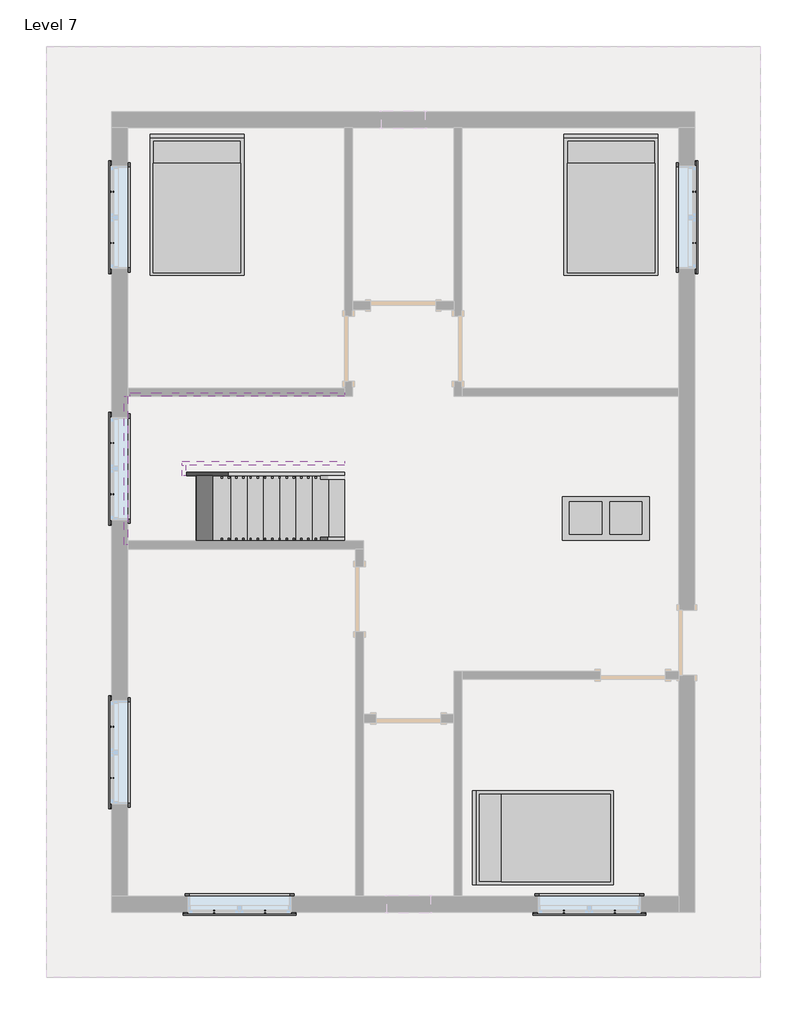
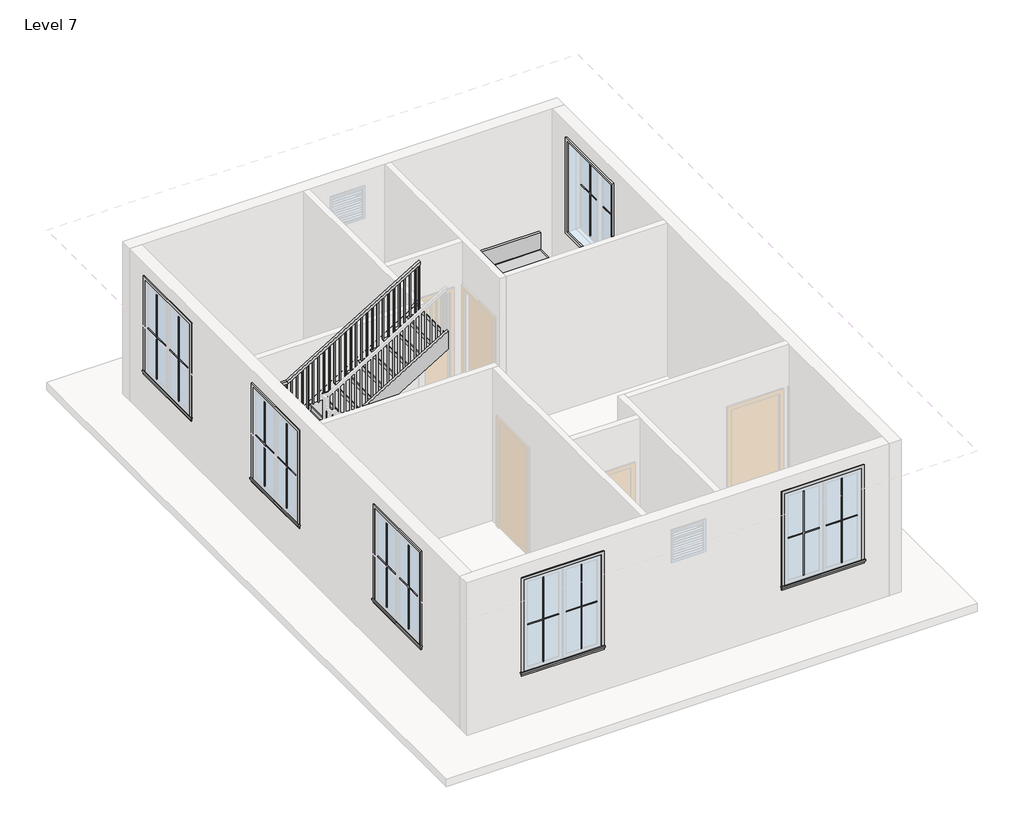
# One storey, part 2 of 2: 25 proxies, 6 members, 3 furniture elements, 1 railing, 1 stair flight.
"""IFC4 building model written with IfcOpenShell, lengths in millimetres."""

from ifc_helpers import new_model, si_unit, frame, origin, place, context, project, spatial, polyline, outline, extrude, faceted_brep, transform, mapped, element, save
from components import muntin_pattern_2x2_muntin_pattern_2x2_bff912c5, muntin_pattern_2x2_muntin_pattern_2x2_c2194282, trim_window_exterior_flat_with_sill_e04b3088, trim_window_interior_flat_picture_frame_2a7685fe, coffee_table_with_brass_mullions_11320_coffee_table_with_5962bef7, bed_17739_bed_17739_15c61121, stair_flight_0d4d62c4

model = new_model("IFC4")

# Units and contexts
model_context = context("Model", 3, world=origin())
ifc_project = project(units=[si_unit("LENGTHUNIT", "METRE", prefix="MILLI")], contexts=[model_context])

# Site, building, storey
site = spatial("IfcSite", under=ifc_project)
building = spatial("IfcBuilding", under=site)
storey = spatial("IfcBuildingStorey", under=building, Name="Level 7", Elevation=16002.0)

# Proxies
placement = place(None, origin())
muntin_pattern_2x2_muntin_pattern_2x2_shape = muntin_pattern_2x2_muntin_pattern_2x2_bff912c5(model_context)
element("IfcBuildingElementProxy", 1, Name="Muntin Pattern_2x2 : Muntin Pattern_2x2", ObjectType="Muntin Pattern_2x2 : Muntin Pattern_2x2", at=placement, inside=storey, context=model_context, shape_type="MappedRepresentation", body=[
    mapped(muntin_pattern_2x2_muntin_pattern_2x2_shape, transform((-3196.8535855, -5792.3946383, 16986.25), x_axis=(-1.0, 0.0, 0.0), y_axis=(0.0, -1.0, 0.0), z_axis=(0.0, 0.0, 1.0))),
])
element("IfcBuildingElementProxy", 2, Name="Muntin Pattern_2x2 : Muntin Pattern_2x2", ObjectType="Muntin Pattern_2x2 : Muntin Pattern_2x2", at=placement, inside=storey, context=model_context, shape_type="MappedRepresentation", body=[
    mapped(muntin_pattern_2x2_muntin_pattern_2x2_shape, transform((-5347.9160855, -3914.3821383, 16986.25), x_axis=(0.0, 1.0, 0.0), y_axis=(-1.0, 0.0, 0.0), z_axis=(0.0, 0.0, 1.0))),
])
element("IfcBuildingElementProxy", 3, Name="Muntin Pattern_2x2 : Muntin Pattern_2x2", ObjectType="Muntin Pattern_2x2 : Muntin Pattern_2x2", at=placement, inside=storey, context=model_context, shape_type="MappedRepresentation", body=[
    mapped(muntin_pattern_2x2_muntin_pattern_2x2_shape, transform((1721.2214145, -5792.3946383, 16986.25), x_axis=(-1.0, 0.0, 0.0), y_axis=(0.0, -1.0, 0.0), z_axis=(0.0, 0.0, 1.0))),
])
element("IfcBuildingElementProxy", 4, Name="Muntin Pattern_2x2 : Muntin Pattern_2x2", ObjectType="Muntin Pattern_2x2 : Muntin Pattern_2x2", at=placement, inside=storey, context=model_context, shape_type="MappedRepresentation", body=[
    mapped(muntin_pattern_2x2_muntin_pattern_2x2_shape, transform((2837.2339145, 4324.7428617, 16986.25), x_axis=(0.0, -1.0, 0.0), y_axis=(1.0, 0.0, 0.0), z_axis=(0.0, 0.0, 1.0))),
])
element("IfcBuildingElementProxy", 5, Name="Muntin Pattern_2x2 : Muntin Pattern_2x2", ObjectType="Muntin Pattern_2x2 : Muntin Pattern_2x2", at=placement, inside=storey, context=model_context, shape_type="MappedRepresentation", body=[
    mapped(muntin_pattern_2x2_muntin_pattern_2x2_shape, transform((-5347.9160855, 3604.0178617, 16986.25), x_axis=(0.0, 1.0, 0.0), y_axis=(-1.0, 0.0, 0.0), z_axis=(0.0, 0.0, 1.0))),
])
element("IfcBuildingElementProxy", 6, Name="Muntin Pattern_2x2 : Muntin Pattern_2x2", ObjectType="Muntin Pattern_2x2 : Muntin Pattern_2x2", at=placement, inside=storey, context=model_context, shape_type="MappedRepresentation", body=[
    mapped(muntin_pattern_2x2_muntin_pattern_2x2_shape, transform((-5347.9160855, 73.4178617, 16986.25), x_axis=(0.0, 1.0, 0.0), y_axis=(-1.0, 0.0, 0.0), z_axis=(0.0, 0.0, 1.0))),
])
muntin_pattern_2x2_muntin_pattern_2x2_2_shape = muntin_pattern_2x2_muntin_pattern_2x2_c2194282(model_context)
element("IfcBuildingElementProxy", 7, Name="Muntin Pattern_2x2 : Muntin Pattern_2x2", ObjectType="Muntin Pattern_2x2 : Muntin Pattern_2x2", at=placement, inside=storey, context=model_context, shape_type="MappedRepresentation", body=[
    mapped(muntin_pattern_2x2_muntin_pattern_2x2_2_shape, transform((-3917.5785855, -5792.3946383, 16986.25), x_axis=(1.0, 0.0, 0.0), y_axis=(0.0, 1.0, 0.0), z_axis=(0.0, 0.0, 1.0))),
])
element("IfcBuildingElementProxy", 8, Name="Muntin Pattern_2x2 : Muntin Pattern_2x2", ObjectType="Muntin Pattern_2x2 : Muntin Pattern_2x2", at=placement, inside=storey, context=model_context, shape_type="MappedRepresentation", body=[
    mapped(muntin_pattern_2x2_muntin_pattern_2x2_2_shape, transform((-5347.9160855, -3193.6571383, 16986.25), x_axis=(0.0, -1.0, 0.0), y_axis=(1.0, 0.0, 0.0), z_axis=(0.0, 0.0, 1.0))),
])
element("IfcBuildingElementProxy", 9, Name="Muntin Pattern_2x2 : Muntin Pattern_2x2", ObjectType="Muntin Pattern_2x2 : Muntin Pattern_2x2", at=placement, inside=storey, context=model_context, shape_type="MappedRepresentation", body=[
    mapped(muntin_pattern_2x2_muntin_pattern_2x2_2_shape, transform((1000.4964145, -5792.3946383, 16986.25), x_axis=(1.0, 0.0, 0.0), y_axis=(0.0, 1.0, 0.0), z_axis=(0.0, 0.0, 1.0))),
])
element("IfcBuildingElementProxy", 10, Name="Muntin Pattern_2x2 : Muntin Pattern_2x2", ObjectType="Muntin Pattern_2x2 : Muntin Pattern_2x2", at=placement, inside=storey, context=model_context, shape_type="MappedRepresentation", body=[
    mapped(muntin_pattern_2x2_muntin_pattern_2x2_2_shape, transform((2837.2339145, 3604.0178617, 16986.25), x_axis=(0.0, 1.0, 0.0), y_axis=(-1.0, 0.0, 0.0), z_axis=(0.0, 0.0, 1.0))),
])
element("IfcBuildingElementProxy", 11, Name="Muntin Pattern_2x2 : Muntin Pattern_2x2", ObjectType="Muntin Pattern_2x2 : Muntin Pattern_2x2", at=placement, inside=storey, context=model_context, shape_type="MappedRepresentation", body=[
    mapped(muntin_pattern_2x2_muntin_pattern_2x2_2_shape, transform((-5347.9160855, 4324.7428617, 16986.25), x_axis=(0.0, -1.0, 0.0), y_axis=(1.0, 0.0, 0.0), z_axis=(0.0, 0.0, 1.0))),
])
element("IfcBuildingElementProxy", 12, Name="Muntin Pattern_2x2 : Muntin Pattern_2x2", ObjectType="Muntin Pattern_2x2 : Muntin Pattern_2x2", at=placement, inside=storey, context=model_context, shape_type="MappedRepresentation", body=[
    mapped(muntin_pattern_2x2_muntin_pattern_2x2_2_shape, transform((-5347.9160855, 794.1428617, 16986.25), x_axis=(0.0, -1.0, 0.0), y_axis=(1.0, 0.0, 0.0), z_axis=(0.0, 0.0, 1.0))),
])
trim_window_exterior_flat_with_sill_shape = trim_window_exterior_flat_with_sill_e04b3088(model_context)
element("IfcBuildingElementProxy", 13, Name="Trim-Window-Exterior-Flat : with Sill", ObjectType="Trim-Window-Exterior-Flat : with Sill", at=placement, inside=storey, context=model_context, shape_type="MappedRepresentation", body=[
    mapped(trim_window_exterior_flat_with_sill_shape, transform((-3557.2160855, -5801.9196383, 18745.2), x_axis=(1.0, 0.0, 0.0), y_axis=(0.0, 0.0, 1.0), z_axis=(0.0, -1.0, 0.0))),
])
element("IfcBuildingElementProxy", 14, Name="Trim-Window-Exterior-Flat : with Sill", ObjectType="Trim-Window-Exterior-Flat : with Sill", at=placement, inside=storey, context=model_context, shape_type="MappedRepresentation", body=[
    mapped(trim_window_exterior_flat_with_sill_shape, transform((-5357.4410855, -3554.0196383, 18745.2), x_axis=(0.0, -1.0, 0.0), y_axis=(0.0, 0.0, 1.0), z_axis=(-1.0, 0.0, 0.0))),
])
element("IfcBuildingElementProxy", 15, Name="Trim-Window-Exterior-Flat : with Sill", ObjectType="Trim-Window-Exterior-Flat : with Sill", at=placement, inside=storey, context=model_context, shape_type="MappedRepresentation", body=[
    mapped(trim_window_exterior_flat_with_sill_shape, transform((1360.8589145, -5801.9196383, 18745.2), x_axis=(1.0, 0.0, 0.0), y_axis=(0.0, 0.0, 1.0), z_axis=(0.0, -1.0, 0.0))),
])
element("IfcBuildingElementProxy", 16, Name="Trim-Window-Exterior-Flat : with Sill", ObjectType="Trim-Window-Exterior-Flat : with Sill", at=placement, inside=storey, context=model_context, shape_type="MappedRepresentation", body=[
    mapped(trim_window_exterior_flat_with_sill_shape, transform((2846.7589145, 3964.3803617, 18745.2), x_axis=(0.0, 1.0, 0.0), y_axis=(0.0, 0.0, 1.0), z_axis=(1.0, 0.0, 0.0))),
])
element("IfcBuildingElementProxy", 17, Name="Trim-Window-Exterior-Flat : with Sill", ObjectType="Trim-Window-Exterior-Flat : with Sill", at=placement, inside=storey, context=model_context, shape_type="MappedRepresentation", body=[
    mapped(trim_window_exterior_flat_with_sill_shape, transform((-5357.4410855, 3964.3803617, 18745.2), x_axis=(0.0, -1.0, 0.0), y_axis=(0.0, 0.0, 1.0), z_axis=(-1.0, 0.0, 0.0))),
])
element("IfcBuildingElementProxy", 18, Name="Trim-Window-Exterior-Flat : with Sill", ObjectType="Trim-Window-Exterior-Flat : with Sill", at=placement, inside=storey, context=model_context, shape_type="MappedRepresentation", body=[
    mapped(trim_window_exterior_flat_with_sill_shape, transform((-5357.4410855, 433.7803617, 18745.2), x_axis=(0.0, -1.0, 0.0), y_axis=(0.0, 0.0, 1.0), z_axis=(-1.0, 0.0, 0.0))),
])
trim_window_interior_flat_picture_frame_shape = trim_window_interior_flat_picture_frame_2a7685fe(model_context)
element("IfcBuildingElementProxy", 19, Name="Trim-Window-Interior-Flat : Picture Frame", ObjectType="Trim-Window-Interior-Flat : Picture Frame", at=placement, inside=storey, context=model_context, shape_type="MappedRepresentation", body=[
    mapped(trim_window_interior_flat_picture_frame_shape, transform((-3557.2160855, -5573.3196383, 18745.2), x_axis=(-1.0, 0.0, 0.0), y_axis=(0.0, 0.0, 1.0), z_axis=(0.0, 1.0, 0.0))),
])
element("IfcBuildingElementProxy", 20, Name="Trim-Window-Interior-Flat : Picture Frame", ObjectType="Trim-Window-Interior-Flat : Picture Frame", at=placement, inside=storey, context=model_context, shape_type="MappedRepresentation", body=[
    mapped(trim_window_interior_flat_picture_frame_shape, transform((-5128.8410855, -3554.0196383, 18745.2), x_axis=(0.0, 1.0, 0.0), y_axis=(0.0, 0.0, 1.0), z_axis=(1.0, 0.0, 0.0))),
])
element("IfcBuildingElementProxy", 21, Name="Trim-Window-Interior-Flat : Picture Frame", ObjectType="Trim-Window-Interior-Flat : Picture Frame", at=placement, inside=storey, context=model_context, shape_type="MappedRepresentation", body=[
    mapped(trim_window_interior_flat_picture_frame_shape, transform((1360.8589145, -5573.3196383, 18745.2), x_axis=(-1.0, 0.0, 0.0), y_axis=(0.0, 0.0, 1.0), z_axis=(0.0, 1.0, 0.0))),
])
element("IfcBuildingElementProxy", 22, Name="Trim-Window-Interior-Flat : Picture Frame", ObjectType="Trim-Window-Interior-Flat : Picture Frame", at=placement, inside=storey, context=model_context, shape_type="MappedRepresentation", body=[
    mapped(trim_window_interior_flat_picture_frame_shape, transform((2618.1589145, 3964.3803617, 18745.2), x_axis=(0.0, -1.0, 0.0), y_axis=(0.0, 0.0, 1.0), z_axis=(-1.0, 0.0, 0.0))),
])
element("IfcBuildingElementProxy", 23, Name="Trim-Window-Interior-Flat : Picture Frame", ObjectType="Trim-Window-Interior-Flat : Picture Frame", at=placement, inside=storey, context=model_context, shape_type="MappedRepresentation", body=[
    mapped(trim_window_interior_flat_picture_frame_shape, transform((-5128.8410855, 3964.3803617, 18745.2), x_axis=(0.0, 1.0, 0.0), y_axis=(0.0, 0.0, 1.0), z_axis=(1.0, 0.0, 0.0))),
])
element("IfcBuildingElementProxy", 24, Name="Trim-Window-Interior-Flat : Picture Frame", ObjectType="Trim-Window-Interior-Flat : Picture Frame", at=placement, inside=storey, context=model_context, shape_type="MappedRepresentation", body=[
    mapped(trim_window_interior_flat_picture_frame_shape, transform((-5128.8410855, 433.7803617, 18745.2), x_axis=(0.0, 1.0, 0.0), y_axis=(0.0, 0.0, 1.0), z_axis=(1.0, 0.0, 0.0))),
])
coffee_table_with_brass_mullions_11320_coffee_table_with_shape = coffee_table_with_brass_mullions_11320_coffee_table_with_5962bef7(model_context)
element("IfcBuildingElementProxy", 25, Name="coffee_table_with_brass_mullions_11320 : coffee_table_with_brass_mullions_11320", ObjectType="coffee_table_with_brass_mullions_11320 : coffee_table_with_brass_mullions_11320", at=placement, inside=storey, context=model_context, shape_type="MappedRepresentation", body=[
    mapped(coffee_table_with_brass_mullions_11320_coffee_table_with_shape, transform((2229.2258874, -696.5196383, 16002.0), x_axis=(1.0, 0.0, 0.0), y_axis=(0.0, 1.0, 0.0), z_axis=(0.0, 0.0, 1.0))),
])

# Furniture
bed_17739_bed_17739_shape = bed_17739_bed_17739_15c61121(model_context)
element("IfcFurniture", 26, ObjectType="Bed_17739 : Bed_17739", at=placement, inside=storey, context=model_context, shape_type="MappedRepresentation", body=[
    mapped(bed_17739_bed_17739_shape, transform((1665.6589145, 4116.7803617, 16002.0), x_axis=(1.0, 0.0, 0.0), y_axis=(0.0, 1.0, 0.0), z_axis=(0.0, 0.0, 1.0))),
])
element("IfcFurniture", 27, ObjectType="Bed_17739 : Bed_17739", at=placement, inside=storey, context=model_context, shape_type="MappedRepresentation", body=[
    mapped(bed_17739_bed_17739_shape, transform((-4157.2910855, 4116.7803617, 16002.0), x_axis=(1.0, 0.0, 0.0), y_axis=(0.0, 1.0, 0.0), z_axis=(0.0, 0.0, 1.0))),
])
element("IfcFurniture", 28, ObjectType="Bed_17739 : Bed_17739", at=placement, inside=storey, context=model_context, shape_type="MappedRepresentation", body=[
    mapped(bed_17739_bed_17739_shape, transform((732.2089145, -4754.5725945, 16002.0), x_axis=(0.0, 1.0, 0.0), y_axis=(-1.0, 0.0, 0.0), z_axis=(0.0, 0.0, 1.0))),
])

# Members
element("IfcMember", 29, ObjectType="Stringer - 2\" Width", at=placement, inside=storey, context=model_context, shape_type="SweptSolid", body=[
    extrude(outline(polyline([(16002.0, -2080.8410855), (16214.114512, -2080.8410855), (17602.2, -4371.1821407), (17602.2, -4959.2565972), (16002.0, -2318.9265972), (16002.0, -2080.8410855)])), frame((0.0, -633.0196383, 0.0), z_axis=(0.0, 1.0, 0.0), x_axis=(0.0, 0.0, 1.0)), (0.0, 0.0, 1.0), 50.8),
])
element("IfcMember", 30, ObjectType="Stringer - 2\" Width", at=placement, inside=storey, context=model_context, shape_type="SweptSolid", body=[
    extrude(outline(polyline([(-5128.8410855, -633.0196383), (-5179.6410855, -633.0196383), (-5179.6410855, 1449.7803617), (-5128.8410855, 1449.7803617), (-5128.8410855, -633.0196383)])), frame((0.0, 0.0, 17297.4), z_axis=(0.0, 0.0, 1.0), x_axis=(1.0, 0.0, 0.0)), (0.0, 0.0, 1.0), 304.8),
])
element("IfcMember", 31, ObjectType="Stringer - 2\" Width", at=placement, inside=storey, context=model_context, shape_type="SweptSolid", body=[
    extrude(outline(polyline([(17297.4, -4505.9455737), (18767.1602959, -2080.8410855), (19123.5690574, -2080.8410855), (17297.4, -5094.0200302), (17297.4, -4505.9455737)])), frame((0.0, 1449.7803617, 0.0), z_axis=(0.0, 1.0, 0.0), x_axis=(0.0, 0.0, 1.0)), (0.0, 0.0, 1.0), 50.8),
])
element("IfcMember", 32, ObjectType="Stringer - 2\" Width", at=placement, inside=storey, context=model_context, shape_type="SweptSolid", body=[
    extrude(outline(polyline([(16002.0, -2080.8410855), (16214.114512, -2080.8410855), (17568.7811786, -4316.0410855), (17212.3724171, -4316.0410855), (16002.0, -2318.9265972), (16002.0, -2080.8410855)])), frame((0.0, 332.1803617, 0.0), z_axis=(0.0, 1.0, 0.0), x_axis=(0.0, 0.0, 1.0)), (0.0, 0.0, 1.0), 50.8),
])
element("IfcMember", 33, ObjectType="Stringer - 2\" Width", at=placement, inside=storey, context=model_context, shape_type="SweptSolid", body=[
    extrude(outline(polyline([(-4316.0410855, 332.1803617), (-4366.8410855, 332.1803617), (-4366.8410855, 484.5803617), (-4316.0410855, 484.5803617), (-4316.0410855, 332.1803617)])), frame((0.0, 0.0, 17297.4), z_axis=(0.0, 0.0, 1.0), x_axis=(1.0, 0.0, 0.0)), (0.0, 0.0, 1.0), 304.8),
])
element("IfcMember", 34, ObjectType="Stringer - 2\" Width", at=placement, inside=storey, context=model_context, shape_type="SweptSolid", body=[
    extrude(outline(polyline([(17738.114512, -4366.8410855), (17381.7057504, -4366.8410855), (18767.1602959, -2080.8410855), (19123.5690574, -2080.8410855), (17738.114512, -4366.8410855)])), frame((0.0, 484.5803617, 0.0), z_axis=(0.0, 1.0, 0.0), x_axis=(0.0, 0.0, 1.0)), (0.0, 0.0, 1.0), 50.8),
])

# Railing
element("IfcRailing", 35, ObjectType="Handrail - Rectangular", at=placement, inside=storey, context=model_context, shape_type="SolidModel", body=[
    faceted_brep([(-2080.8410855, -582.2196383, 17054.9454545), (-2080.8410855, -582.2196383, 16995.5439943), (-2080.8410855, -531.4196383, 16995.5439943), (-2080.8410855, -531.4196383, 17054.9454545), (-4366.8410855, -582.2196383, 18440.4), (-4381.0334949, -582.2196383, 18389.6), (-4381.0334949, -531.4196383, 18389.6), (-4366.8410855, -531.4196383, 18440.4), (-5128.8410855, -582.2196383, 18440.4), (-5128.8410855, -582.2196383, 18389.6), (-5078.0410855, -531.4196383, 18389.6), (-5078.0410855, -531.4196383, 18440.4), (-5128.8410855, 1449.7803617, 18440.4), (-5128.8410855, 1449.7803617, 18389.6), (-5078.0410855, 1398.9803617, 18389.6), (-5078.0410855, 1398.9803617, 18440.4), (-4595.4410855, 1449.7803617, 18440.4), (-4581.2486761, 1449.7803617, 18389.6), (-4581.2486761, 1398.9803617, 18389.6), (-4595.4410855, 1398.9803617, 18440.4), (-2080.8410855, 1449.7803617, 19964.4), (-2080.8410855, 1398.9803617, 19964.4), (-2080.8410855, 1398.9803617, 19904.9985397), (-2080.8410855, 1449.7803617, 19904.9985397)], [[[0, 1, 2, 3]], [[1, 0, 4, 5]], [[2, 1, 5, 6]], [[3, 2, 6, 7]], [[0, 3, 7, 4]], [[5, 4, 8, 9]], [[6, 5, 9, 10]], [[7, 6, 10, 11]], [[4, 7, 11, 8]], [[9, 8, 12, 13]], [[10, 9, 13, 14]], [[11, 10, 14, 15]], [[8, 11, 15, 12]], [[13, 12, 16, 17]], [[14, 13, 17, 18]], [[15, 14, 18, 19]], [[12, 15, 19, 16]], [[20, 21, 22, 23]], [[17, 16, 20, 23]], [[18, 17, 23, 22]], [[19, 18, 22, 21]], [[16, 19, 21, 20]]]),
    extrude(outline(polyline([(19853.0439943, -2166.5660855), (18911.4545455, -2166.5660855), (18911.4545455, -2147.5160855), (19864.5894488, -2147.5160855), (19853.0439943, -2166.5660855)])), frame((0.0, 1414.8553617, 0.0), z_axis=(0.0, 1.0, 0.0), x_axis=(0.0, 0.0, 1.0)), (0.0, 0.0, 1.0), 19.05),
    extrude(outline(polyline([(19791.4682367, -2268.1660855), (18911.4545455, -2268.1660855), (18911.4545455, -2249.1160855), (19803.0136913, -2249.1160855), (19791.4682367, -2268.1660855)])), frame((0.0, 1414.8553617, 0.0), z_axis=(0.0, 1.0, 0.0), x_axis=(0.0, 0.0, 1.0)), (0.0, 0.0, 1.0), 19.05),
    extrude(outline(polyline([(19729.8924791, -2369.7660855), (18772.9090909, -2369.7660855), (18772.9090909, -2350.7160855), (19741.4379337, -2350.7160855), (19729.8924791, -2369.7660855)])), frame((0.0, 1414.8553617, 0.0), z_axis=(0.0, 1.0, 0.0), x_axis=(0.0, 0.0, 1.0)), (0.0, 0.0, 1.0), 19.05),
    extrude(outline(polyline([(19668.3167216, -2471.3660855), (18772.9090909, -2471.3660855), (18772.9090909, -2452.3160855), (19679.8621761, -2452.3160855), (19668.3167216, -2471.3660855)])), frame((0.0, 1414.8553617, 0.0), z_axis=(0.0, 1.0, 0.0), x_axis=(0.0, 0.0, 1.0)), (0.0, 0.0, 1.0), 19.05),
    extrude(outline(polyline([(19606.740964, -2572.9660855), (18634.3636364, -2572.9660855), (18634.3636364, -2553.9160855), (19618.2864185, -2553.9160855), (19606.740964, -2572.9660855)])), frame((0.0, 1414.8553617, 0.0), z_axis=(0.0, 1.0, 0.0), x_axis=(0.0, 0.0, 1.0)), (0.0, 0.0, 1.0), 19.05),
    extrude(outline(polyline([(19545.1652064, -2674.5660855), (18634.3636364, -2674.5660855), (18634.3636364, -2655.5160855), (19556.710661, -2655.5160855), (19545.1652064, -2674.5660855)])), frame((0.0, 1414.8553617, 0.0), z_axis=(0.0, 1.0, 0.0), x_axis=(0.0, 0.0, 1.0)), (0.0, 0.0, 1.0), 19.05),
    extrude(outline(polyline([(19483.5894488, -2776.1660855), (18634.3636364, -2776.1660855), (18634.3636364, -2757.1160855), (19495.1349034, -2757.1160855), (19483.5894488, -2776.1660855)])), frame((0.0, 1414.8553617, 0.0), z_axis=(0.0, 1.0, 0.0), x_axis=(0.0, 0.0, 1.0)), (0.0, 0.0, 1.0), 19.05),
    extrude(outline(polyline([(19422.0136913, -2877.7660855), (18495.8181818, -2877.7660855), (18495.8181818, -2858.7160855), (19433.5591458, -2858.7160855), (19422.0136913, -2877.7660855)])), frame((0.0, 1414.8553617, 0.0), z_axis=(0.0, 1.0, 0.0), x_axis=(0.0, 0.0, 1.0)), (0.0, 0.0, 1.0), 19.05),
    extrude(outline(polyline([(19360.4379337, -2979.3660855), (18495.8181818, -2979.3660855), (18495.8181818, -2960.3160855), (19371.9833882, -2960.3160855), (19360.4379337, -2979.3660855)])), frame((0.0, 1414.8553617, 0.0), z_axis=(0.0, 1.0, 0.0), x_axis=(0.0, 0.0, 1.0)), (0.0, 0.0, 1.0), 19.05),
    extrude(outline(polyline([(19298.8621761, -3080.9660855), (18357.2727273, -3080.9660855), (18357.2727273, -3061.9160855), (19310.4076307, -3061.9160855), (19298.8621761, -3080.9660855)])), frame((0.0, 1414.8553617, 0.0), z_axis=(0.0, 1.0, 0.0), x_axis=(0.0, 0.0, 1.0)), (0.0, 0.0, 1.0), 19.05),
    extrude(outline(polyline([(19237.2864185, -3182.5660855), (18357.2727273, -3182.5660855), (18357.2727273, -3163.5160855), (19248.8318731, -3163.5160855), (19237.2864185, -3182.5660855)])), frame((0.0, 1414.8553617, 0.0), z_axis=(0.0, 1.0, 0.0), x_axis=(0.0, 0.0, 1.0)), (0.0, 0.0, 1.0), 19.05),
    extrude(outline(polyline([(19175.710661, -3284.1660855), (18218.7272727, -3284.1660855), (18218.7272727, -3265.1160855), (19187.2561155, -3265.1160855), (19175.710661, -3284.1660855)])), frame((0.0, 1414.8553617, 0.0), z_axis=(0.0, 1.0, 0.0), x_axis=(0.0, 0.0, 1.0)), (0.0, 0.0, 1.0), 19.05),
    extrude(outline(polyline([(19114.1349034, -3385.7660855), (18218.7272727, -3385.7660855), (18218.7272727, -3366.7160855), (19125.6803579, -3366.7160855), (19114.1349034, -3385.7660855)])), frame((0.0, 1414.8553617, 0.0), z_axis=(0.0, 1.0, 0.0), x_axis=(0.0, 0.0, 1.0)), (0.0, 0.0, 1.0), 19.05),
    extrude(outline(polyline([(19052.5591458, -3487.3660855), (18080.1818182, -3487.3660855), (18080.1818182, -3468.3160855), (19064.1046004, -3468.3160855), (19052.5591458, -3487.3660855)])), frame((0.0, 1414.8553617, 0.0), z_axis=(0.0, 1.0, 0.0), x_axis=(0.0, 0.0, 1.0)), (0.0, 0.0, 1.0), 19.05),
    extrude(outline(polyline([(18990.9833882, -3588.9660855), (18080.1818182, -3588.9660855), (18080.1818182, -3569.9160855), (19002.5288428, -3569.9160855), (18990.9833882, -3588.9660855)])), frame((0.0, 1414.8553617, 0.0), z_axis=(0.0, 1.0, 0.0), x_axis=(0.0, 0.0, 1.0)), (0.0, 0.0, 1.0), 19.05),
    extrude(outline(polyline([(18929.4076307, -3690.5660855), (18080.1818182, -3690.5660855), (18080.1818182, -3671.5160855), (18940.9530852, -3671.5160855), (18929.4076307, -3690.5660855)])), frame((0.0, 1414.8553617, 0.0), z_axis=(0.0, 1.0, 0.0), x_axis=(0.0, 0.0, 1.0)), (0.0, 0.0, 1.0), 19.05),
    extrude(outline(polyline([(18867.8318731, -3792.1660855), (17941.6363636, -3792.1660855), (17941.6363636, -3773.1160855), (18879.3773276, -3773.1160855), (18867.8318731, -3792.1660855)])), frame((0.0, 1414.8553617, 0.0), z_axis=(0.0, 1.0, 0.0), x_axis=(0.0, 0.0, 1.0)), (0.0, 0.0, 1.0), 19.05),
    extrude(outline(polyline([(18806.2561155, -3893.7660855), (17941.6363636, -3893.7660855), (17941.6363636, -3874.7160855), (18817.80157, -3874.7160855), (18806.2561155, -3893.7660855)])), frame((0.0, 1414.8553617, 0.0), z_axis=(0.0, 1.0, 0.0), x_axis=(0.0, 0.0, 1.0)), (0.0, 0.0, 1.0), 19.05),
    extrude(outline(polyline([(18744.6803579, -3995.3660855), (17803.0909091, -3995.3660855), (17803.0909091, -3976.3160855), (18756.2258125, -3976.3160855), (18744.6803579, -3995.3660855)])), frame((0.0, 1414.8553617, 0.0), z_axis=(0.0, 1.0, 0.0), x_axis=(0.0, 0.0, 1.0)), (0.0, 0.0, 1.0), 19.05),
    extrude(outline(polyline([(18683.1046004, -4096.9660855), (17803.0909091, -4096.9660855), (17803.0909091, -4077.9160855), (18694.6500549, -4077.9160855), (18683.1046004, -4096.9660855)])), frame((0.0, 1414.8553617, 0.0), z_axis=(0.0, 1.0, 0.0), x_axis=(0.0, 0.0, 1.0)), (0.0, 0.0, 1.0), 19.05),
    extrude(outline(polyline([(18621.5288428, -4198.5660855), (17664.5454545, -4198.5660855), (17664.5454545, -4179.5160855), (18633.0742973, -4179.5160855), (18621.5288428, -4198.5660855)])), frame((0.0, 1414.8553617, 0.0), z_axis=(0.0, 1.0, 0.0), x_axis=(0.0, 0.0, 1.0)), (0.0, 0.0, 1.0), 19.05),
    extrude(outline(polyline([(18559.9530852, -4300.1660855), (17664.5454545, -4300.1660855), (17664.5454545, -4281.1160855), (18571.4985397, -4281.1160855), (18559.9530852, -4300.1660855)])), frame((0.0, 1414.8553617, 0.0), z_axis=(0.0, 1.0, 0.0), x_axis=(0.0, 0.0, 1.0)), (0.0, 0.0, 1.0), 19.05),
    extrude(outline(polyline([(18498.3773276, -4401.7660855), (17526.0, -4401.7660855), (17526.0, -4382.7160855), (18509.9227822, -4382.7160855), (18498.3773276, -4401.7660855)])), frame((0.0, 1414.8553617, 0.0), z_axis=(0.0, 1.0, 0.0), x_axis=(0.0, 0.0, 1.0)), (0.0, 0.0, 1.0), 19.05),
    extrude(outline(polyline([(18436.80157, -4503.3660855), (17526.0, -4503.3660855), (17526.0, -4484.3160855), (18448.3470246, -4484.3160855), (18436.80157, -4503.3660855)])), frame((0.0, 1414.8553617, 0.0), z_axis=(0.0, 1.0, 0.0), x_axis=(0.0, 0.0, 1.0)), (0.0, 0.0, 1.0), 19.05),
    extrude(outline(polyline([(-4604.9660855, 1433.9053617), (-4585.9160855, 1433.9053617), (-4585.9160855, 1414.8553617), (-4604.9660855, 1414.8553617), (-4604.9660855, 1433.9053617)])), frame((0.0, 0.0, 17526.0), z_axis=(0.0, 0.0, 1.0), x_axis=(1.0, 0.0, 0.0)), (0.0, 0.0, 1.0), 863.6),
    extrude(outline(polyline([(-4706.5660855, 1433.9053617), (-4687.5160855, 1433.9053617), (-4687.5160855, 1414.8553617), (-4706.5660855, 1414.8553617), (-4706.5660855, 1433.9053617)])), frame((0.0, 0.0, 17526.0), z_axis=(0.0, 0.0, 1.0), x_axis=(1.0, 0.0, 0.0)), (0.0, 0.0, 1.0), 863.6),
    extrude(outline(polyline([(-4808.1660855, 1433.9053617), (-4789.1160855, 1433.9053617), (-4789.1160855, 1414.8553617), (-4808.1660855, 1414.8553617), (-4808.1660855, 1433.9053617)])), frame((0.0, 0.0, 17526.0), z_axis=(0.0, 0.0, 1.0), x_axis=(1.0, 0.0, 0.0)), (0.0, 0.0, 1.0), 863.6),
    extrude(outline(polyline([(-4909.7660855, 1433.9053617), (-4890.7160855, 1433.9053617), (-4890.7160855, 1414.8553617), (-4909.7660855, 1414.8553617), (-4909.7660855, 1433.9053617)])), frame((0.0, 0.0, 17526.0), z_axis=(0.0, 0.0, 1.0), x_axis=(1.0, 0.0, 0.0)), (0.0, 0.0, 1.0), 863.6),
    extrude(outline(polyline([(-5011.3660855, 1433.9053617), (-4992.3160855, 1433.9053617), (-4992.3160855, 1414.8553617), (-5011.3660855, 1414.8553617), (-5011.3660855, 1433.9053617)])), frame((0.0, 0.0, 17526.0), z_axis=(0.0, 0.0, 1.0), x_axis=(1.0, 0.0, 0.0)), (0.0, 0.0, 1.0), 863.6),
    extrude(outline(polyline([(-5112.9660855, 1364.0553617), (-5112.9660855, 1383.1053617), (-5093.9160855, 1383.1053617), (-5093.9160855, 1364.0553617), (-5112.9660855, 1364.0553617)])), frame((0.0, 0.0, 17526.0), z_axis=(0.0, 0.0, 1.0), x_axis=(1.0, 0.0, 0.0)), (0.0, 0.0, 1.0), 863.6),
    extrude(outline(polyline([(-5112.9660855, 1262.4553617), (-5112.9660855, 1281.5053617), (-5093.9160855, 1281.5053617), (-5093.9160855, 1262.4553617), (-5112.9660855, 1262.4553617)])), frame((0.0, 0.0, 17526.0), z_axis=(0.0, 0.0, 1.0), x_axis=(1.0, 0.0, 0.0)), (0.0, 0.0, 1.0), 863.6),
    extrude(outline(polyline([(-5112.9660855, 1160.8553617), (-5112.9660855, 1179.9053617), (-5093.9160855, 1179.9053617), (-5093.9160855, 1160.8553617), (-5112.9660855, 1160.8553617)])), frame((0.0, 0.0, 17526.0), z_axis=(0.0, 0.0, 1.0), x_axis=(1.0, 0.0, 0.0)), (0.0, 0.0, 1.0), 863.6),
    extrude(outline(polyline([(-5112.9660855, 1059.2553617), (-5112.9660855, 1078.3053617), (-5093.9160855, 1078.3053617), (-5093.9160855, 1059.2553617), (-5112.9660855, 1059.2553617)])), frame((0.0, 0.0, 17526.0), z_axis=(0.0, 0.0, 1.0), x_axis=(1.0, 0.0, 0.0)), (0.0, 0.0, 1.0), 863.6),
    extrude(outline(polyline([(-5112.9660855, 957.6553617), (-5112.9660855, 976.7053617), (-5093.9160855, 976.7053617), (-5093.9160855, 957.6553617), (-5112.9660855, 957.6553617)])), frame((0.0, 0.0, 17526.0), z_axis=(0.0, 0.0, 1.0), x_axis=(1.0, 0.0, 0.0)), (0.0, 0.0, 1.0), 863.6),
    extrude(outline(polyline([(-5112.9660855, 856.0553617), (-5112.9660855, 875.1053617), (-5093.9160855, 875.1053617), (-5093.9160855, 856.0553617), (-5112.9660855, 856.0553617)])), frame((0.0, 0.0, 17526.0), z_axis=(0.0, 0.0, 1.0), x_axis=(1.0, 0.0, 0.0)), (0.0, 0.0, 1.0), 863.6),
    extrude(outline(polyline([(-5112.9660855, 754.4553617), (-5112.9660855, 773.5053617), (-5093.9160855, 773.5053617), (-5093.9160855, 754.4553617), (-5112.9660855, 754.4553617)])), frame((0.0, 0.0, 17526.0), z_axis=(0.0, 0.0, 1.0), x_axis=(1.0, 0.0, 0.0)), (0.0, 0.0, 1.0), 863.6),
    extrude(outline(polyline([(-5112.9660855, 652.8553617), (-5112.9660855, 671.9053617), (-5093.9160855, 671.9053617), (-5093.9160855, 652.8553617), (-5112.9660855, 652.8553617)])), frame((0.0, 0.0, 17526.0), z_axis=(0.0, 0.0, 1.0), x_axis=(1.0, 0.0, 0.0)), (0.0, 0.0, 1.0), 863.6),
    extrude(outline(polyline([(-5112.9660855, 551.2553617), (-5112.9660855, 570.3053617), (-5093.9160855, 570.3053617), (-5093.9160855, 551.2553617), (-5112.9660855, 551.2553617)])), frame((0.0, 0.0, 17526.0), z_axis=(0.0, 0.0, 1.0), x_axis=(1.0, 0.0, 0.0)), (0.0, 0.0, 1.0), 863.6),
    extrude(outline(polyline([(-5112.9660855, 449.6553617), (-5112.9660855, 468.7053617), (-5093.9160855, 468.7053617), (-5093.9160855, 449.6553617), (-5112.9660855, 449.6553617)])), frame((0.0, 0.0, 17526.0), z_axis=(0.0, 0.0, 1.0), x_axis=(1.0, 0.0, 0.0)), (0.0, 0.0, 1.0), 863.6),
    extrude(outline(polyline([(-5112.9660855, 348.0553617), (-5112.9660855, 367.1053617), (-5093.9160855, 367.1053617), (-5093.9160855, 348.0553617), (-5112.9660855, 348.0553617)])), frame((0.0, 0.0, 17526.0), z_axis=(0.0, 0.0, 1.0), x_axis=(1.0, 0.0, 0.0)), (0.0, 0.0, 1.0), 863.6),
    extrude(outline(polyline([(-5112.9660855, 246.4553617), (-5112.9660855, 265.5053617), (-5093.9160855, 265.5053617), (-5093.9160855, 246.4553617), (-5112.9660855, 246.4553617)])), frame((0.0, 0.0, 17526.0), z_axis=(0.0, 0.0, 1.0), x_axis=(1.0, 0.0, 0.0)), (0.0, 0.0, 1.0), 863.6),
    extrude(outline(polyline([(-5112.9660855, 144.8553617), (-5112.9660855, 163.9053617), (-5093.9160855, 163.9053617), (-5093.9160855, 144.8553617), (-5112.9660855, 144.8553617)])), frame((0.0, 0.0, 17526.0), z_axis=(0.0, 0.0, 1.0), x_axis=(1.0, 0.0, 0.0)), (0.0, 0.0, 1.0), 863.6),
    extrude(outline(polyline([(-5112.9660855, 43.2553617), (-5112.9660855, 62.3053617), (-5093.9160855, 62.3053617), (-5093.9160855, 43.2553617), (-5112.9660855, 43.2553617)])), frame((0.0, 0.0, 17526.0), z_axis=(0.0, 0.0, 1.0), x_axis=(1.0, 0.0, 0.0)), (0.0, 0.0, 1.0), 863.6),
    extrude(outline(polyline([(-5112.9660855, -58.3446383), (-5112.9660855, -39.2946383), (-5093.9160855, -39.2946383), (-5093.9160855, -58.3446383), (-5112.9660855, -58.3446383)])), frame((0.0, 0.0, 17526.0), z_axis=(0.0, 0.0, 1.0), x_axis=(1.0, 0.0, 0.0)), (0.0, 0.0, 1.0), 863.6),
    extrude(outline(polyline([(-5112.9660855, -159.9446383), (-5112.9660855, -140.8946383), (-5093.9160855, -140.8946383), (-5093.9160855, -159.9446383), (-5112.9660855, -159.9446383)])), frame((0.0, 0.0, 17526.0), z_axis=(0.0, 0.0, 1.0), x_axis=(1.0, 0.0, 0.0)), (0.0, 0.0, 1.0), 863.6),
    extrude(outline(polyline([(-5112.9660855, -261.5446383), (-5112.9660855, -242.4946383), (-5093.9160855, -242.4946383), (-5093.9160855, -261.5446383), (-5112.9660855, -261.5446383)])), frame((0.0, 0.0, 17526.0), z_axis=(0.0, 0.0, 1.0), x_axis=(1.0, 0.0, 0.0)), (0.0, 0.0, 1.0), 863.6),
    extrude(outline(polyline([(-5112.9660855, -363.1446383), (-5112.9660855, -344.0946383), (-5093.9160855, -344.0946383), (-5093.9160855, -363.1446383), (-5112.9660855, -363.1446383)])), frame((0.0, 0.0, 17526.0), z_axis=(0.0, 0.0, 1.0), x_axis=(1.0, 0.0, 0.0)), (0.0, 0.0, 1.0), 863.6),
    extrude(outline(polyline([(-5112.9660855, -464.7446383), (-5112.9660855, -445.6946383), (-5093.9160855, -445.6946383), (-5093.9160855, -464.7446383), (-5112.9660855, -464.7446383)])), frame((0.0, 0.0, 17526.0), z_axis=(0.0, 0.0, 1.0), x_axis=(1.0, 0.0, 0.0)), (0.0, 0.0, 1.0), 863.6),
    extrude(outline(polyline([(-5017.7160855, -566.3446383), (-5036.7660855, -566.3446383), (-5036.7660855, -547.2946383), (-5017.7160855, -547.2946383), (-5017.7160855, -566.3446383)])), frame((0.0, 0.0, 17526.0), z_axis=(0.0, 0.0, 1.0), x_axis=(1.0, 0.0, 0.0)), (0.0, 0.0, 1.0), 863.6),
    extrude(outline(polyline([(-4916.1160855, -566.3446383), (-4935.1660855, -566.3446383), (-4935.1660855, -547.2946383), (-4916.1160855, -547.2946383), (-4916.1160855, -566.3446383)])), frame((0.0, 0.0, 17526.0), z_axis=(0.0, 0.0, 1.0), x_axis=(1.0, 0.0, 0.0)), (0.0, 0.0, 1.0), 863.6),
    extrude(outline(polyline([(-4814.5160855, -566.3446383), (-4833.5660855, -566.3446383), (-4833.5660855, -547.2946383), (-4814.5160855, -547.2946383), (-4814.5160855, -566.3446383)])), frame((0.0, 0.0, 17526.0), z_axis=(0.0, 0.0, 1.0), x_axis=(1.0, 0.0, 0.0)), (0.0, 0.0, 1.0), 863.6),
    extrude(outline(polyline([(-4712.9160855, -566.3446383), (-4731.9660855, -566.3446383), (-4731.9660855, -547.2946383), (-4712.9160855, -547.2946383), (-4712.9160855, -566.3446383)])), frame((0.0, 0.0, 17526.0), z_axis=(0.0, 0.0, 1.0), x_axis=(1.0, 0.0, 0.0)), (0.0, 0.0, 1.0), 863.6),
    extrude(outline(polyline([(-4611.3160855, -566.3446383), (-4630.3660855, -566.3446383), (-4630.3660855, -547.2946383), (-4611.3160855, -547.2946383), (-4611.3160855, -566.3446383)])), frame((0.0, 0.0, 17526.0), z_axis=(0.0, 0.0, 1.0), x_axis=(1.0, 0.0, 0.0)), (0.0, 0.0, 1.0), 863.6),
    extrude(outline(polyline([(-4509.7160855, -566.3446383), (-4528.7660855, -566.3446383), (-4528.7660855, -547.2946383), (-4509.7160855, -547.2946383), (-4509.7160855, -566.3446383)])), frame((0.0, 0.0, 17526.0), z_axis=(0.0, 0.0, 1.0), x_axis=(1.0, 0.0, 0.0)), (0.0, 0.0, 1.0), 863.6),
    extrude(outline(polyline([(-4408.1160855, -566.3446383), (-4427.1660855, -566.3446383), (-4427.1660855, -547.2946383), (-4408.1160855, -547.2946383), (-4408.1160855, -566.3446383)])), frame((0.0, 0.0, 17526.0), z_axis=(0.0, 0.0, 1.0), x_axis=(1.0, 0.0, 0.0)), (0.0, 0.0, 1.0), 863.6),
    extrude(outline(polyline([(18355.9833882, -4325.5660855), (17387.4545455, -4325.5660855), (17387.4545455, -4306.5160855), (18344.4379337, -4306.5160855), (18355.9833882, -4325.5660855)])), frame((0.0, -566.3446383, 0.0), z_axis=(0.0, 1.0, 0.0), x_axis=(0.0, 0.0, 1.0)), (0.0, 0.0, 1.0), 19.05),
    extrude(outline(polyline([(18294.4076307, -4223.9660855), (17387.4545455, -4223.9660855), (17387.4545455, -4204.9160855), (18282.8621761, -4204.9160855), (18294.4076307, -4223.9660855)])), frame((0.0, -566.3446383, 0.0), z_axis=(0.0, 1.0, 0.0), x_axis=(0.0, 0.0, 1.0)), (0.0, 0.0, 1.0), 19.05),
    extrude(outline(polyline([(18232.8318731, -4122.3660855), (17248.9090909, -4122.3660855), (17248.9090909, -4103.3160855), (18221.2864185, -4103.3160855), (18232.8318731, -4122.3660855)])), frame((0.0, -566.3446383, 0.0), z_axis=(0.0, 1.0, 0.0), x_axis=(0.0, 0.0, 1.0)), (0.0, 0.0, 1.0), 19.05),
    extrude(outline(polyline([(18171.2561155, -4020.7660855), (17248.9090909, -4020.7660855), (17248.9090909, -4001.7160855), (18159.710661, -4001.7160855), (18171.2561155, -4020.7660855)])), frame((0.0, -566.3446383, 0.0), z_axis=(0.0, 1.0, 0.0), x_axis=(0.0, 0.0, 1.0)), (0.0, 0.0, 1.0), 19.05),
    extrude(outline(polyline([(18109.6803579, -3919.1660855), (17248.9090909, -3919.1660855), (17248.9090909, -3900.1160855), (18098.1349034, -3900.1160855), (18109.6803579, -3919.1660855)])), frame((0.0, -566.3446383, 0.0), z_axis=(0.0, 1.0, 0.0), x_axis=(0.0, 0.0, 1.0)), (0.0, 0.0, 1.0), 19.05),
    extrude(outline(polyline([(18048.1046004, -3817.5660855), (17110.3636364, -3817.5660855), (17110.3636364, -3798.5160855), (18036.5591458, -3798.5160855), (18048.1046004, -3817.5660855)])), frame((0.0, -566.3446383, 0.0), z_axis=(0.0, 1.0, 0.0), x_axis=(0.0, 0.0, 1.0)), (0.0, 0.0, 1.0), 19.05),
    extrude(outline(polyline([(17986.5288428, -3715.9660855), (17110.3636364, -3715.9660855), (17110.3636364, -3696.9160855), (17974.9833882, -3696.9160855), (17986.5288428, -3715.9660855)])), frame((0.0, -566.3446383, 0.0), z_axis=(0.0, 1.0, 0.0), x_axis=(0.0, 0.0, 1.0)), (0.0, 0.0, 1.0), 19.05),
    extrude(outline(polyline([(17924.9530852, -3614.3660855), (16971.8181818, -3614.3660855), (16971.8181818, -3595.3160855), (17913.4076307, -3595.3160855), (17924.9530852, -3614.3660855)])), frame((0.0, -566.3446383, 0.0), z_axis=(0.0, 1.0, 0.0), x_axis=(0.0, 0.0, 1.0)), (0.0, 0.0, 1.0), 19.05),
    extrude(outline(polyline([(17863.3773276, -3512.7660855), (16971.8181818, -3512.7660855), (16971.8181818, -3493.7160855), (17851.8318731, -3493.7160855), (17863.3773276, -3512.7660855)])), frame((0.0, -566.3446383, 0.0), z_axis=(0.0, 1.0, 0.0), x_axis=(0.0, 0.0, 1.0)), (0.0, 0.0, 1.0), 19.05),
    extrude(outline(polyline([(17801.80157, -3411.1660855), (16833.2727273, -3411.1660855), (16833.2727273, -3392.1160855), (17790.2561155, -3392.1160855), (17801.80157, -3411.1660855)])), frame((0.0, -566.3446383, 0.0), z_axis=(0.0, 1.0, 0.0), x_axis=(0.0, 0.0, 1.0)), (0.0, 0.0, 1.0), 19.05),
    extrude(outline(polyline([(17740.2258125, -3309.5660855), (16833.2727273, -3309.5660855), (16833.2727273, -3290.5160855), (17728.6803579, -3290.5160855), (17740.2258125, -3309.5660855)])), frame((0.0, -566.3446383, 0.0), z_axis=(0.0, 1.0, 0.0), x_axis=(0.0, 0.0, 1.0)), (0.0, 0.0, 1.0), 19.05),
    extrude(outline(polyline([(17678.6500549, -3207.9660855), (16694.7272727, -3207.9660855), (16694.7272727, -3188.9160855), (17667.1046004, -3188.9160855), (17678.6500549, -3207.9660855)])), frame((0.0, -566.3446383, 0.0), z_axis=(0.0, 1.0, 0.0), x_axis=(0.0, 0.0, 1.0)), (0.0, 0.0, 1.0), 19.05),
    extrude(outline(polyline([(17617.0742973, -3106.3660855), (16694.7272727, -3106.3660855), (16694.7272727, -3087.3160855), (17605.5288428, -3087.3160855), (17617.0742973, -3106.3660855)])), frame((0.0, -566.3446383, 0.0), z_axis=(0.0, 1.0, 0.0), x_axis=(0.0, 0.0, 1.0)), (0.0, 0.0, 1.0), 19.05),
    extrude(outline(polyline([(17555.4985397, -3004.7660855), (16694.7272727, -3004.7660855), (16694.7272727, -2985.7160855), (17543.9530852, -2985.7160855), (17555.4985397, -3004.7660855)])), frame((0.0, -566.3446383, 0.0), z_axis=(0.0, 1.0, 0.0), x_axis=(0.0, 0.0, 1.0)), (0.0, 0.0, 1.0), 19.05),
    extrude(outline(polyline([(17493.9227822, -2903.1660855), (16556.1818182, -2903.1660855), (16556.1818182, -2884.1160855), (17482.3773276, -2884.1160855), (17493.9227822, -2903.1660855)])), frame((0.0, -566.3446383, 0.0), z_axis=(0.0, 1.0, 0.0), x_axis=(0.0, 0.0, 1.0)), (0.0, 0.0, 1.0), 19.05),
    extrude(outline(polyline([(17432.3470246, -2801.5660855), (16556.1818182, -2801.5660855), (16556.1818182, -2782.5160855), (17420.80157, -2782.5160855), (17432.3470246, -2801.5660855)])), frame((0.0, -566.3446383, 0.0), z_axis=(0.0, 1.0, 0.0), x_axis=(0.0, 0.0, 1.0)), (0.0, 0.0, 1.0), 19.05),
    extrude(outline(polyline([(17370.771267, -2699.9660855), (16417.6363636, -2699.9660855), (16417.6363636, -2680.9160855), (17359.2258125, -2680.9160855), (17370.771267, -2699.9660855)])), frame((0.0, -566.3446383, 0.0), z_axis=(0.0, 1.0, 0.0), x_axis=(0.0, 0.0, 1.0)), (0.0, 0.0, 1.0), 19.05),
    extrude(outline(polyline([(17309.1955094, -2598.3660855), (16417.6363636, -2598.3660855), (16417.6363636, -2579.3160855), (17297.6500549, -2579.3160855), (17309.1955094, -2598.3660855)])), frame((0.0, -566.3446383, 0.0), z_axis=(0.0, 1.0, 0.0), x_axis=(0.0, 0.0, 1.0)), (0.0, 0.0, 1.0), 19.05),
    extrude(outline(polyline([(17247.6197519, -2496.7660855), (16279.0909091, -2496.7660855), (16279.0909091, -2477.7160855), (17236.0742973, -2477.7160855), (17247.6197519, -2496.7660855)])), frame((0.0, -566.3446383, 0.0), z_axis=(0.0, 1.0, 0.0), x_axis=(0.0, 0.0, 1.0)), (0.0, 0.0, 1.0), 19.05),
    extrude(outline(polyline([(17186.0439943, -2395.1660855), (16279.0909091, -2395.1660855), (16279.0909091, -2376.1160855), (17174.4985397, -2376.1160855), (17186.0439943, -2395.1660855)])), frame((0.0, -566.3446383, 0.0), z_axis=(0.0, 1.0, 0.0), x_axis=(0.0, 0.0, 1.0)), (0.0, 0.0, 1.0), 19.05),
    extrude(outline(polyline([(17124.4682367, -2293.5660855), (16140.5454545, -2293.5660855), (16140.5454545, -2274.5160855), (17112.9227822, -2274.5160855), (17124.4682367, -2293.5660855)])), frame((0.0, -566.3446383, 0.0), z_axis=(0.0, 1.0, 0.0), x_axis=(0.0, 0.0, 1.0)), (0.0, 0.0, 1.0), 19.05),
    extrude(outline(polyline([(17062.8924791, -2191.9660855), (16140.5454545, -2191.9660855), (16140.5454545, -2172.9160855), (17051.3470246, -2172.9160855), (17062.8924791, -2191.9660855)])), frame((0.0, -566.3446383, 0.0), z_axis=(0.0, 1.0, 0.0), x_axis=(0.0, 0.0, 1.0)), (0.0, 0.0, 1.0), 19.05),
    extrude(outline(polyline([(-5112.9660855, 1414.8553617), (-5112.9660855, 1433.9053617), (-5093.9160855, 1433.9053617), (-5093.9160855, 1414.8553617), (-5112.9660855, 1414.8553617)])), frame((0.0, 0.0, 17526.0), z_axis=(0.0, 0.0, 1.0), x_axis=(1.0, 0.0, 0.0)), (0.0, 0.0, 1.0), 863.6),
    extrude(outline(polyline([(-5093.9160855, -566.3446383), (-5112.9660855, -566.3446383), (-5112.9660855, -547.2946383), (-5093.9160855, -547.2946383), (-5093.9160855, -566.3446383)])), frame((0.0, 0.0, 17526.0), z_axis=(0.0, 0.0, 1.0), x_axis=(1.0, 0.0, 0.0)), (0.0, 0.0, 1.0), 863.6),
    extrude(outline(polyline([(19893.4530852, -2099.8910855), (18911.4545455, -2099.8910855), (18911.4545455, -2080.8410855), (19904.9985397, -2080.8410855), (19893.4530852, -2099.8910855)])), frame((0.0, 1414.8553617, 0.0), z_axis=(0.0, 1.0, 0.0), x_axis=(0.0, 0.0, 1.0)), (0.0, 0.0, 1.0), 19.05),
    extrude(outline(polyline([(17007.0894488, -2099.8910855), (16140.5454545, -2099.8910855), (16140.5454545, -2080.8410855), (16995.5439943, -2080.8410855), (17007.0894488, -2099.8910855)])), frame((0.0, -566.3446383, 0.0), z_axis=(0.0, 1.0, 0.0), x_axis=(0.0, 0.0, 1.0)), (0.0, 0.0, 1.0), 19.05),
])

# Stair flight
stair_flight_shape = stair_flight_0d4d62c4(model_context)
element("IfcStairFlight", 36, ObjectType="2\" Tread 1\" Nosing 1/4\" Riser", at=placement, inside=storey, context=model_context, shape_type="MappedRepresentation", body=[
    mapped(stair_flight_shape, transform((0.0, 0.0, 0.0), x_axis=(1.0, 0.0, 0.0), y_axis=(0.0, 1.0, 0.0), z_axis=(0.0, 0.0, 1.0))),
])

save(model, "model.ifc")

# Revit data of these elements
# Type "Muntin Pattern_2x2 : Muntin Pattern_2x2"
#   Width [instance default] = 4' - 0"
#   Thickness = 0' - 0 1/2"
#   Height [instance default] = 4' - 0"
#   Distance = 0' - 0 3/4"
#   Interior Material [instance default] = none
#   Exterior Material [instance default] = none
#   Default Elevation = 0
# Type "Trim-Window-Exterior-Flat : with Sill"
#   Trim Width = 0' - 2 1/4"
#   Trim Thickness_Picture Frame = 0' - 1 1/4"
#   Trim Thickness_with Sill = 0' - 0 3/4"
#   Sill Thickness = 0' - 1 1/4"
#   Opening Width [instance default] = 2' - 0"
#   Opening Height [instance default] = 3' - 0"
#   Default Elevation = 4' - 0"
#   Sill = yes
#   Picture Frame = no
#   Trim Material [instance default] = none
# Type "Trim-Window-Interior-Flat : Picture Frame"
#   Trim Thickness_Picture Frame = 0' - 1 1/4"
#   Trim Width = 0' - 2 1/4"
#   Trim Thickness_with Sill = 0' - 0 3/4"
#   Sill Thickness = 0' - 1 1/4"
#   Opening Width [instance default] = 2' - 0"
#   Opening Height [instance default] = 3' - 0"
#   Default Elevation = 4' - 0"
#   Sill = no
#   Picture Frame = yes
#   Trim Material [instance default] = none
# Type "coffee_table_with_brass_mullions_11320 : coffee_table_with_brass_mullions_11320"
#   Default Elevation = 0
# Type "Bed_17739 : Bed_17739"
#   Default Elevation = 0
# Type "Handrail - Rectangular"
#   Assembly Code = "C2010400"
#   built-in parameter 1008612 = 0.0416667 (stored number, unit not read)
#   built-in parameter 1008611 = 0.0416667 (stored number, unit not read)
#   built-in parameter 1008609 = 0.333333 (stored number, unit not read)
#   built-in parameter 1008604 = 0.166667 (stored number, unit not read)
#   built-in parameter 1008603 = 0.166667 (stored number, unit not read)
#   Railing Height = 3' - 0"
#   built-in parameter 1008630 = 2
#   built-in parameter 1008610 = 2
#   built-in parameter 1008618 = Baluster - Square : 3/4"
# Elements 1, 2, 3, 4, 5, 6, 7, 8, 9, 10, 11, 12 (IfcBuildingElementProxy, "Muntin Pattern_2x2 : Muntin Pattern_2x2")
#   Width = 1' - 11 1/8"
#   Height = 5' - 6 1/2"
#   Interior Material = Wood - Stained
#   Exterior Material = Clad - White
#   Phase Created = New Construction
#   Materials on its faces: "Clad - White", "Wood - Stained"
# Elements 13, 14, 15, 16, 17, 18 (IfcBuildingElementProxy, "Trim-Window-Exterior-Flat : with Sill")
#   Opening Width = 4' - 9"
#   Opening Height = 6' - 0"
#   Trim Material = Clad - White
#   Phase Created = New Construction
#   Materials on its faces: "Clad - White"
# Elements 19, 20, 21, 22, 23, 24 (IfcBuildingElementProxy, "Trim-Window-Interior-Flat : Picture Frame")
#   Opening Width = 4' - 9"
#   Opening Height = 6' - 0"
#   Trim Material = Wood - Stained
#   Phase Created = New Construction
#   Materials on its faces: "Wood - Stained"
# Element 25 (IfcBuildingElementProxy, "coffee_table_with_brass_mullions_11320 : coffee_table_with_brass_mullions_11320")
#   Phase Created = New Construction
#   Materials on its faces: "Default Wall", "TABLE", "Glass", "Default"
# Elements 26, 27, 28 (IfcFurniture, "Bed_17739 : Bed_17739")
#   Phase Created = New Construction
#   Materials on its faces: "legs", "sheets", "bed frame", "Blanket"
# Elements 29, 30, 31, 32, 33, 34 (IfcMember, "Stringer - 2\" Width")
#   Phase Created = New Construction
# Element 35 (IfcRailing, "Handrail - Rectangular")
#   Phase Created = New Construction
# Element 36 (IfcStairFlight, "2\" Tread 1\" Nosing 1/4\" Riser")
#   Phase Created = New Construction
# Materials
#   "Clad - White": class "Wood", colour RGB 242 242 238, transparency 0, Cost = 0
#   "Wood - Stained": class "Wood", colour RGB 224 178 126, transparency 0, Cost = 0
#   "Default Wall": colour RGB 128 128 128, transparency 0, Cost = 0
#   "TABLE": class "Generic", colour RGB 120 120 120, transparency 0, Cost = 0
#   "Glass": class "Glass", colour RGB 0 128 192, transparency 0.75, Description = "Soda Lime Glass", Cost = 0
#   "Default": colour RGB 127 127 127, transparency 0, Cost = 0
#   "legs": colour RGB 90 73 37, transparency 0, Cost = 0
#   "sheets": colour RGB 200 195 176, transparency 0, Cost = 0
#   "bed frame": colour RGB 90 73 37, transparency 0, Cost = 0
#   "Blanket": class "System", colour RGB 59 0 1, transparency 0, Cost = 0
